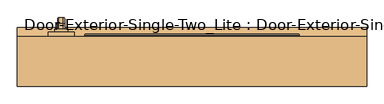
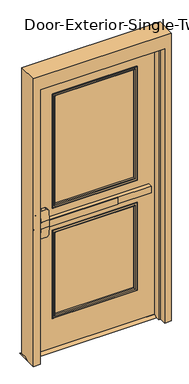
"""IFC4 building model written with IfcOpenShell, lengths in millimetres: door geometry, Door-Exterior-Single-Two_Lite : Door-Exterior-Single-Two_Lite."""

from ifc_helpers import new_model, si_unit, point, frame, frame_2d, origin, place, context, project, spatial, polyline, circle_curve, ellipse_curve, trimmed, segment, composite_curve, outline, extrude, faceted_brep, source, transform, mapped, element, save
from ifc_brep_helpers import plane_surface, cylinder_surface, revolved_surface, advanced_brep


def door_exterior_single_two_lite_door_exterior_single_two_lite_36a17ea7(model_context):
    return source(origin(), model_context, "Body", "SolidModel", [
        extrude(outline(polyline([(38.1, 12.7), (82.55, 12.7), (107.95, 0.0), (12.7, 0.0), (38.1, 12.7)])), frame((-508.0, 0.0, 0.0), z_axis=(1.0, 0.0, 0.0), x_axis=(0.0, 1.0, 0.0)), (0.0, 0.0, 1.0), 1016.0),
        extrude(outline(polyline([(150.2833333, 0.0), (-349.25, 0.0), (-349.25, 6.35), (150.2833333, 6.35), (150.2833333, 0.0)])), frame((0.0, 0.0, 990.6), z_axis=(0.0, 0.0, 1.0), x_axis=(1.0, 0.0, 0.0)), (0.0, 0.0, 1.0), 50.8),
        advanced_brep(
        [(-412.75, 6.35, 1041.4), (-412.75, 6.35, 990.6), (-349.25, 6.35, 990.6), (400.05, 6.35, 990.6), (400.05, 6.35, 1041.4), (-349.25, 6.35, 1041.4), (400.05, 38.1, 1041.4), (400.05, 38.1, 990.6), (-349.25, 38.1, 990.6), (-349.25, 38.1, 927.1), (-368.3, 38.1, 908.05), (-393.7, 38.1, 908.05), (-412.75, 38.1, 927.1), (-412.75, 38.1, 1104.9), (-393.7, 38.1, 1123.95), (-368.3, 38.1, 1123.95), (-349.25, 38.1, 1104.9), (-349.25, 38.1, 1041.4), (-349.25, 9.5252467, 1041.4), (-412.75, 9.5252467, 1041.4), (-412.75, 14.5354269, 1104.9), (-412.75, 14.5354269, 927.1), (-412.75, 9.5252467, 990.6), (-349.25, 9.5252467, 990.6), (-349.25, 14.5354269, 927.1), (-349.25, 14.5354269, 1104.9), (-393.7, 16.038481, 1123.95), (-368.3, 16.038481, 1123.95), (-368.3, 16.038481, 908.05), (-393.7, 16.038481, 908.05)],
        [
            (0, 1),
            (1, 2),
            (2, 3),
            (3, 4),
            (4, 5),
            (5, 0),
            (6, 7),
            (7, 8),
            (8, 9),
            (9, 10, circle_curve(frame((-368.3, 38.1, 927.1), z_axis=(0.0, 1.0, 0.0), x_axis=(1.0, 0.0, 0.0)), 19.05)),
            (10, 11),
            (11, 12, circle_curve(frame((-393.7, 38.1, 927.1), z_axis=(0.0, 1.0, 0.0), x_axis=(1.0, 0.0, 0.0)), 19.05)),
            (12, 13),
            (13, 14, circle_curve(frame((-393.7, 38.1, 1104.9), z_axis=(0.0, 1.0, 0.0), x_axis=(1.0, 0.0, 0.0)), 19.05)),
            (14, 15),
            (15, 16, circle_curve(frame((-368.3, 38.1, 1104.9), z_axis=(0.0, 1.0, 0.0), x_axis=(1.0, 0.0, 0.0)), 19.05)),
            (16, 17),
            (17, 6),
            (4, 6),
            (17, 18),
            (18, 19),
            (19, 0),
            (19, 20),
            (20, 13),
            (12, 21),
            (21, 22),
            (22, 1),
            (7, 3),
            (22, 23),
            (23, 8),
            (23, 24),
            (24, 9),
            (16, 25),
            (25, 18),
            (14, 26),
            (26, 27),
            (27, 15),
            (10, 28),
            (28, 29),
            (29, 11),
            (24, 28, ellipse_curve(frame((-368.3, 14.5354269, 927.1), z_axis=(0.0, 0.9969018152893365, 0.07865602756830282), x_axis=(0.0, -0.07865602756830208, 0.9969018152893365)), 19.1092038, 19.05)),
            (27, 25, ellipse_curve(frame((-368.3, 14.5354269, 1104.9), z_axis=(0.0, 0.9969018152893376, -0.07865602756828934), x_axis=(0.0, -0.078656027568288, -0.9969018152893377)), 19.1092038, 19.05)),
            (20, 26, ellipse_curve(frame((-393.7, 14.5354269, 1104.9), z_axis=(0.0, 0.9969018152893376, -0.07865602756828934), x_axis=(0.0, -0.078656027568288, -0.9969018152893377)), 19.1092038, 19.05)),
            (29, 21, ellipse_curve(frame((-393.7, 14.5354269, 927.1), z_axis=(0.0, 0.9969018152893365, 0.07865602756830282), x_axis=(0.0, -0.07865602756830208, 0.9969018152893365)), 19.1092038, 19.05)),
        ],
        [
            plane_surface(frame((-412.75, 6.35, 1041.4), z_axis=(0.0, -1.0, 0.0), x_axis=(-1.0, 0.0, 0.0))),
            plane_surface(frame((-412.75, 38.1, 1041.4), z_axis=(0.0, 1.0, 0.0), x_axis=(1.0, 0.0, 0.0))),
            plane_surface(frame((400.05, 6.35, 1041.4), z_axis=(0.0, 0.0, 1.0), x_axis=(0.0, 1.0, 0.0))),
            plane_surface(frame((-412.75, 6.35, 1041.4), z_axis=(-1.0, 0.0, 0.0), x_axis=(0.0, 1.0, 0.0))),
            plane_surface(frame((-412.75, 6.35, 990.6), z_axis=(0.0, 0.0, -1.0), x_axis=(0.0, 1.0, 0.0))),
            plane_surface(frame((400.05, 6.35, 990.6), z_axis=(1.0, 0.0, 0.0), x_axis=(0.0, 1.0, 0.0))),
            plane_surface(frame((-349.25, 9.5252467, 927.1), z_axis=(1.0, 0.0, 0.0), x_axis=(0.0, 1.0, 0.0))),
            plane_surface(frame((-368.3, 9.5252467, 1123.95), z_axis=(0.0, 0.0, 1.0), x_axis=(0.0, 1.0, 0.0))),
            plane_surface(frame((-393.7, 9.5252467, 908.05), z_axis=(0.0, 0.0, -1.0), x_axis=(0.0, 1.0, 0.0))),
            cylinder_surface(frame((-368.3, 38.1, 927.1), z_axis=(0.0, -1.0, 0.0), x_axis=(1.0, 0.0, 0.0)), 19.05),
            cylinder_surface(frame((-368.3, 38.1, 1104.9), z_axis=(0.0, -1.0, 0.0), x_axis=(1.0, 0.0, 0.0)), 19.05),
            cylinder_surface(frame((-393.7, 38.1, 1104.9), z_axis=(0.0, -1.0, 0.0), x_axis=(1.0, 0.0, 0.0)), 19.05),
            cylinder_surface(frame((-393.7, 38.1, 927.1), z_axis=(0.0, -1.0, 0.0), x_axis=(1.0, 0.0, 0.0)), 19.05),
            plane_surface(frame((-349.25, 9.5252467, 1041.4), z_axis=(0.0, -0.9969018152893376, 0.07865602756828934), x_axis=(-1.0, 0.0, 0.0))),
            plane_surface(frame((-349.25, 16.038481, 908.05), z_axis=(0.0, -0.9969018152893365, -0.07865602756830282), x_axis=(-1.0, 0.0, 0.0))),
        ],
        [
            (0, [[1, 2, 3, 4, 5, 6]]),
            (1, [[7, 8, 9, 10, 11, 12, 13, 14, 15, 16, 17, 18]]),
            (2, [[19, -18, 20, 21, 22, -6, -5]]),
            (3, [[-1, -22, 23, 24, -13, 25, 26, 27]]),
            (4, [[28, -3, -2, -27, 29, 30, -8]]),
            (5, [[-4, -28, -7, -19]]),
            (6, [[-9, -30, 31, 32]]),
            (6, [[-17, 33, 34, -20]]),
            (7, [[-15, 35, 36, 37]]),
            (8, [[-11, 38, 39, 40]]),
            (9, [[-10, -32, 41, -38]]),
            (10, [[-16, -37, 42, -33]]),
            (11, [[-14, -24, 43, -35]]),
            (12, [[-12, -40, 44, -25]]),
            (13, [[-21, -34, -42, -36, -43, -23]]),
            (14, [[-26, -44, -39, -41, -31, -29]]),
        ],
    ),
        advanced_brep(
        [(-391.0, 95.25, 1017.190625), (-391.0, 95.25, 1014.809375), (-387.428125, 95.25, 1011.2375), (-374.5715406, 95.25, 1011.2375), (-371.0, 95.25, 1014.8090406), (-371.0, 95.25, 1017.190625), (-374.571875, 95.25, 1020.7625), (-387.428125, 95.25, 1020.7625), (-391.0, 95.25, 887.809375), (-387.428125, 95.25, 884.2375), (-374.571875, 95.25, 884.2375), (-371.0, 95.25, 887.809375), (-371.0, 95.25, 890.1909594), (-374.5715406, 95.25, 893.7625), (-387.428125, 95.25, 893.7625), (-391.0, 95.25, 890.190625), (-391.0, 120.65, 1017.190625), (-391.0, 134.540625, 1003.3), (-391.0, 134.540625, 901.7), (-391.0, 120.65, 887.809375), (-391.0, 120.65, 890.190625), (-391.0, 132.159375, 901.7), (-391.0, 132.159375, 1003.3), (-391.0, 120.65, 1014.809375), (-387.428125, 120.65, 1011.2375), (-374.5715406, 120.65, 1011.2375), (-371.0, 120.65, 1014.8090406), (-371.0, 132.1590406, 1003.3), (-371.0, 132.1590406, 901.7), (-371.0, 120.65, 890.1909594), (-371.0, 120.65, 887.809375), (-371.0, 134.540625, 901.7), (-371.0, 134.540625, 1003.3), (-371.0, 120.65, 1017.190625), (-374.571875, 120.65, 1020.7625), (-387.428125, 120.65, 1020.7625), (-387.428125, 128.5875, 1003.3), (-374.5715406, 128.5875, 1003.3), (-374.571875, 138.1125, 1003.3), (-387.428125, 138.1125, 1003.3), (-387.428125, 128.5875, 901.7), (-374.5715406, 128.5875, 901.7), (-374.571875, 138.1125, 901.7), (-387.428125, 138.1125, 901.7), (-387.428125, 120.65, 893.7625), (-374.5715406, 120.65, 893.7625), (-374.571875, 120.65, 884.2375), (-387.428125, 120.65, 884.2375)],
        [
            (0, 1),
            (1, 2, circle_curve(frame((-387.428125, 95.25, 1014.809375), z_axis=(0.0, -1.0, 0.0), x_axis=(0.0, 0.0, 1.0)), 3.571875)),
            (2, 3),
            (3, 4, circle_curve(frame((-374.5715406, 95.25, 1014.8090406), z_axis=(0.0, -1.0, 0.0), x_axis=(0.0, 0.0, 1.0)), 3.5715406)),
            (4, 5),
            (5, 6, circle_curve(frame((-374.571875, 95.25, 1017.190625), z_axis=(0.0, -1.0, 0.0), x_axis=(0.0, 0.0, 1.0)), 3.571875)),
            (6, 7),
            (7, 0, circle_curve(frame((-387.428125, 95.25, 1017.190625), z_axis=(0.0, -1.0, 0.0), x_axis=(0.0, 0.0, 1.0)), 3.571875)),
            (8, 9, circle_curve(frame((-387.428125, 95.25, 887.809375), z_axis=(0.0, -1.0, 0.0), x_axis=(0.0, 0.0, -1.0)), 3.571875)),
            (9, 10),
            (10, 11, circle_curve(frame((-374.571875, 95.25, 887.809375), z_axis=(0.0, -1.0, 0.0), x_axis=(0.0, 0.0, -1.0)), 3.571875)),
            (11, 12),
            (12, 13, circle_curve(frame((-374.5715406, 95.25, 890.1909594), z_axis=(0.0, -1.0, 0.0), x_axis=(0.0, 0.0, -1.0)), 3.5715406)),
            (13, 14),
            (14, 15, circle_curve(frame((-387.428125, 95.25, 890.190625), z_axis=(0.0, -1.0, 0.0), x_axis=(0.0, 0.0, -1.0)), 3.571875)),
            (15, 8),
            (0, 16),
            (16, 17, circle_curve(frame((-391.0, 120.65, 1003.3), z_axis=(-1.0, 0.0, 0.0), x_axis=(0.0, 0.0, 1.0)), 13.890625)),
            (17, 18),
            (18, 19, circle_curve(frame((-391.0, 120.65, 901.7), z_axis=(-1.0, 0.0, 0.0), x_axis=(0.0, 1.0, 0.0)), 13.890625)),
            (19, 8),
            (15, 20),
            (20, 21, circle_curve(frame((-391.0, 120.65, 901.7), z_axis=(1.0, 0.0, 0.0), x_axis=(0.0, 1.0, 0.0)), 11.509375)),
            (21, 22),
            (22, 23, circle_curve(frame((-391.0, 120.65, 1003.3), z_axis=(1.0, 0.0, 0.0), x_axis=(0.0, 0.0, 1.0)), 11.509375)),
            (23, 1),
            (23, 24, circle_curve(frame((-387.428125, 120.65, 1014.809375), z_axis=(0.0, -1.0, 0.0), x_axis=(0.0, 0.0, 1.0)), 3.571875)),
            (24, 2),
            (24, 25),
            (25, 3),
            (25, 26, circle_curve(frame((-374.5715406, 120.65, 1014.8090406), z_axis=(0.0, -1.0, 0.0), x_axis=(0.0, 0.0, 1.0)), 3.5715406)),
            (26, 4),
            (26, 27, circle_curve(frame((-371.0, 120.65, 1003.3), z_axis=(-1.0, 0.0, 0.0), x_axis=(0.0, 0.0, 1.0)), 11.5090406)),
            (27, 28),
            (28, 29, circle_curve(frame((-371.0, 120.65, 901.7), z_axis=(-1.0, 0.0, 0.0), x_axis=(0.0, 1.0, 0.0)), 11.5090406)),
            (29, 12),
            (11, 30),
            (30, 31, circle_curve(frame((-371.0, 120.65, 901.7), z_axis=(1.0, 0.0, 0.0), x_axis=(0.0, 1.0, 0.0)), 13.890625)),
            (31, 32),
            (32, 33, circle_curve(frame((-371.0, 120.65, 1003.3), z_axis=(1.0, 0.0, 0.0), x_axis=(0.0, 0.0, 1.0)), 13.890625)),
            (33, 5),
            (33, 34, circle_curve(frame((-374.571875, 120.65, 1017.190625), z_axis=(0.0, -1.0, 0.0), x_axis=(0.0, 0.0, 1.0)), 3.571875)),
            (34, 6),
            (34, 35),
            (35, 7),
            (35, 16, circle_curve(frame((-387.428125, 120.65, 1017.190625), z_axis=(0.0, -1.0, 0.0), x_axis=(0.0, 0.0, 1.0)), 3.571875)),
            (36, 24, circle_curve(frame((-387.428125, 120.65, 1003.3), z_axis=(1.0, 0.0, 0.0), x_axis=(0.0, 0.0, 1.0)), 7.9375)),
            (22, 36, circle_curve(frame((-387.428125, 132.159375, 1003.3), z_axis=(0.0, 0.0, 1.0), x_axis=(0.0, 1.0, 0.0)), 3.571875)),
            (37, 25, circle_curve(frame((-374.5715406, 120.65, 1003.3), z_axis=(1.0, 0.0, 0.0), x_axis=(0.0, 0.0, 1.0)), 7.9375)),
            (36, 37),
            (37, 27, circle_curve(frame((-374.5715406, 132.1590406, 1003.3), z_axis=(0.0, 0.0, 1.0), x_axis=(0.0, 1.0, 0.0)), 3.5715406)),
            (38, 34, circle_curve(frame((-374.571875, 120.65, 1003.3), z_axis=(1.0, 0.0, 0.0), x_axis=(0.0, 0.0, 1.0)), 17.4625)),
            (32, 38, circle_curve(frame((-374.571875, 134.540625, 1003.3), z_axis=(0.0, 0.0, 1.0), x_axis=(0.0, 1.0, 0.0)), 3.571875)),
            (39, 35, circle_curve(frame((-387.428125, 120.65, 1003.3), z_axis=(1.0, 0.0, 0.0), x_axis=(0.0, 0.0, 1.0)), 17.4625)),
            (38, 39),
            (39, 17, circle_curve(frame((-387.428125, 134.540625, 1003.3), z_axis=(0.0, 0.0, 1.0), x_axis=(0.0, 1.0, 0.0)), 3.571875)),
            (21, 40, circle_curve(frame((-387.428125, 132.159375, 901.7), z_axis=(0.0, 0.0, 1.0), x_axis=(0.0, 1.0, 0.0)), 3.571875)),
            (40, 36),
            (40, 41),
            (41, 37),
            (41, 28, circle_curve(frame((-374.5715406, 132.1590406, 901.7), z_axis=(0.0, 0.0, 1.0), x_axis=(0.0, 1.0, 0.0)), 3.5715406)),
            (31, 42, circle_curve(frame((-374.571875, 134.540625, 901.7), z_axis=(0.0, 0.0, 1.0), x_axis=(0.0, 1.0, 0.0)), 3.571875)),
            (42, 38),
            (42, 43),
            (43, 39),
            (43, 18, circle_curve(frame((-387.428125, 134.540625, 901.7), z_axis=(0.0, 0.0, 1.0), x_axis=(0.0, 1.0, 0.0)), 3.571875)),
            (44, 40, circle_curve(frame((-387.428125, 120.65, 901.7), z_axis=(1.0, 0.0, 0.0), x_axis=(0.0, 1.0, 0.0)), 7.9375)),
            (20, 44, circle_curve(frame((-387.428125, 120.65, 890.190625), z_axis=(0.0, 1.0, 0.0), x_axis=(0.0, 0.0, -1.0)), 3.571875)),
            (45, 41, circle_curve(frame((-374.5715406, 120.65, 901.7), z_axis=(1.0, 0.0, 0.0), x_axis=(0.0, 1.0, 0.0)), 7.9375)),
            (44, 45),
            (45, 29, circle_curve(frame((-374.5715406, 120.65, 890.1909594), z_axis=(0.0, 1.0, 0.0), x_axis=(0.0, 0.0, -1.0)), 3.5715406)),
            (46, 42, circle_curve(frame((-374.571875, 120.65, 901.7), z_axis=(1.0, 0.0, 0.0), x_axis=(0.0, 1.0, 0.0)), 17.4625)),
            (30, 46, circle_curve(frame((-374.571875, 120.65, 887.809375), z_axis=(0.0, 1.0, 0.0), x_axis=(0.0, 0.0, -1.0)), 3.571875)),
            (47, 43, circle_curve(frame((-387.428125, 120.65, 901.7), z_axis=(1.0, 0.0, 0.0), x_axis=(0.0, 1.0, 0.0)), 17.4625)),
            (46, 47),
            (47, 19, circle_curve(frame((-387.428125, 120.65, 887.809375), z_axis=(0.0, 1.0, 0.0), x_axis=(0.0, 0.0, -1.0)), 3.571875)),
            (14, 44),
            (13, 45),
            (10, 46),
            (9, 47),
        ],
        [
            plane_surface(frame((-381.0, 95.25, 1016.0), z_axis=(0.0, -1.0, 0.0), x_axis=(1.0, 0.0, 0.0))),
            plane_surface(frame((-381.0, 95.25, 889.0), z_axis=(0.0, -1.0, 0.0), x_axis=(1.0, 0.0, 0.0))),
            plane_surface(frame((-391.0, 95.25, 1017.190625), z_axis=(-1.0, 0.0, 0.0), x_axis=(0.0, 1.0, 0.0))),
            cylinder_surface(frame((-387.428125, 95.25, 1014.809375), z_axis=(0.0, -1.0, 0.0), x_axis=(0.0, 0.0, 1.0)), 3.571875),
            plane_surface(frame((-387.428125, 95.25, 1011.2375), z_axis=(0.0, 0.0, -1.0), x_axis=(0.0, 1.0, 0.0))),
            cylinder_surface(frame((-374.5715406, 95.25, 1014.8090406), z_axis=(0.0, -1.0, 0.0), x_axis=(0.0, 0.0, 1.0)), 3.5715406),
            plane_surface(frame((-371.0, 95.25, 1014.8090406), z_axis=(1.0, 0.0, 0.0), x_axis=(0.0, 1.0, 0.0))),
            cylinder_surface(frame((-374.571875, 95.25, 1017.190625), z_axis=(0.0, -1.0, 0.0), x_axis=(0.0, 0.0, 1.0)), 3.571875),
            plane_surface(frame((-374.571875, 95.25, 1020.7625), z_axis=(0.0, 0.0, 1.0), x_axis=(0.0, 1.0, 0.0))),
            cylinder_surface(frame((-387.428125, 95.25, 1017.190625), z_axis=(0.0, -1.0, 0.0), x_axis=(0.0, 0.0, 1.0)), 3.571875),
            revolved_surface(trimmed(ellipse_curve(frame((-387.428125, 120.65, 1014.809375), z_axis=(0.0, -1.0, 0.0), x_axis=(0.0, 0.0, 1.0)), 3.571875, 3.571875), [point((-391.0, 120.65, 1014.809375))], [point((-387.428125, 120.65, 1011.2375))], True, "CARTESIAN"), (-381.0, 120.65, 1003.3), (-1.0, 0.0, 0.0)),
            revolved_surface(polyline([(-387.428125, 120.65, 1011.2375), (-374.5715406, 120.65, 1011.2375)]), (-381.0, 120.65, 1003.3), (-1.0, 0.0, 0.0)),
            revolved_surface(trimmed(ellipse_curve(frame((-374.5715406, 120.65, 1014.8090406), z_axis=(0.0, -1.0, 0.0), x_axis=(0.0, 0.0, 1.0)), 3.5715406, 3.5715406), [point((-374.5715406, 120.65, 1011.2375))], [point((-371.0, 120.65, 1014.8090406))], True, "CARTESIAN"), (-381.0, 120.65, 1003.3), (-1.0, 0.0, 0.0)),
            revolved_surface(trimmed(ellipse_curve(frame((-374.571875, 120.65, 1017.190625), z_axis=(0.0, -1.0, 0.0), x_axis=(0.0, 0.0, 1.0)), 3.571875, 3.571875), [point((-371.0, 120.65, 1017.190625))], [point((-374.571875, 120.65, 1020.7625))], True, "CARTESIAN"), (-381.0, 120.65, 1003.3), (-1.0, 0.0, 0.0)),
            cylinder_surface(frame((-381.0, 120.65, 1003.3), z_axis=(-1.0, 0.0, 0.0), x_axis=(0.0, 0.0, 1.0)), 17.4625),
            revolved_surface(trimmed(ellipse_curve(frame((-387.428125, 120.65, 1017.190625), z_axis=(0.0, -1.0, 0.0), x_axis=(0.0, 0.0, 1.0)), 3.571875, 3.571875), [point((-387.428125, 120.65, 1020.7625))], [point((-391.0, 120.65, 1017.190625))], True, "CARTESIAN"), (-381.0, 120.65, 1003.3), (-1.0, 0.0, 0.0)),
            cylinder_surface(frame((-387.428125, 132.159375, 1003.3), z_axis=(0.0, 0.0, 1.0), x_axis=(0.0, 1.0, 0.0)), 3.571875),
            plane_surface(frame((-387.428125, 128.5875, 1003.3), z_axis=(0.0, -1.0, 0.0), x_axis=(0.0, 0.0, -1.0))),
            cylinder_surface(frame((-374.5715406, 132.1590406, 1003.3), z_axis=(0.0, 0.0, 1.0), x_axis=(0.0, 1.0, 0.0)), 3.5715406),
            cylinder_surface(frame((-374.571875, 134.540625, 1003.3), z_axis=(0.0, 0.0, 1.0), x_axis=(0.0, 1.0, 0.0)), 3.571875),
            plane_surface(frame((-374.571875, 138.1125, 1003.3), z_axis=(0.0, 1.0, 0.0), x_axis=(0.0, 0.0, -1.0))),
            cylinder_surface(frame((-387.428125, 134.540625, 1003.3), z_axis=(0.0, 0.0, 1.0), x_axis=(0.0, 1.0, 0.0)), 3.571875),
            revolved_surface(trimmed(ellipse_curve(frame((-387.428125, 132.159375, 901.7), z_axis=(0.0, 0.0, 1.0), x_axis=(0.0, 1.0, 0.0)), 3.571875, 3.571875), [point((-391.0, 132.159375, 901.7))], [point((-387.428125, 128.5875, 901.7))], True, "CARTESIAN"), (-381.0, 120.65, 901.7), (-1.0, 0.0, 0.0)),
            revolved_surface(polyline([(-387.428125, 128.5875, 901.7), (-374.5715406, 128.5875, 901.7)]), (-381.0, 120.65, 901.7), (-1.0, 0.0, 0.0)),
            revolved_surface(trimmed(ellipse_curve(frame((-374.5715406, 132.1590406, 901.7), z_axis=(0.0, 0.0, 1.0), x_axis=(0.0, 1.0, 0.0)), 3.5715406, 3.5715406), [point((-374.5715406, 128.5875, 901.7))], [point((-371.0, 132.1590406, 901.7))], True, "CARTESIAN"), (-381.0, 120.65, 901.7), (-1.0, 0.0, 0.0)),
            revolved_surface(trimmed(ellipse_curve(frame((-374.571875, 134.540625, 901.7), z_axis=(0.0, 0.0, 1.0), x_axis=(0.0, 1.0, 0.0)), 3.571875, 3.571875), [point((-371.0, 134.540625, 901.7))], [point((-374.571875, 138.1125, 901.7))], True, "CARTESIAN"), (-381.0, 120.65, 901.7), (-1.0, 0.0, 0.0)),
            cylinder_surface(frame((-381.0, 120.65, 901.7), z_axis=(-1.0, 0.0, 0.0), x_axis=(0.0, 1.0, 0.0)), 17.4625),
            revolved_surface(trimmed(ellipse_curve(frame((-387.428125, 134.540625, 901.7), z_axis=(0.0, 0.0, 1.0), x_axis=(0.0, 1.0, 0.0)), 3.571875, 3.571875), [point((-387.428125, 138.1125, 901.7))], [point((-391.0, 134.540625, 901.7))], True, "CARTESIAN"), (-381.0, 120.65, 901.7), (-1.0, 0.0, 0.0)),
            cylinder_surface(frame((-387.428125, 120.65, 890.190625), z_axis=(0.0, 1.0, 0.0), x_axis=(0.0, 0.0, -1.0)), 3.571875),
            plane_surface(frame((-387.428125, 120.65, 893.7625), z_axis=(0.0, 0.0, 1.0), x_axis=(0.0, -1.0, 0.0))),
            cylinder_surface(frame((-374.5715406, 120.65, 890.1909594), z_axis=(0.0, 1.0, 0.0), x_axis=(0.0, 0.0, -1.0)), 3.5715406),
            cylinder_surface(frame((-374.571875, 120.65, 887.809375), z_axis=(0.0, 1.0, 0.0), x_axis=(0.0, 0.0, -1.0)), 3.571875),
            plane_surface(frame((-374.571875, 120.65, 884.2375), z_axis=(0.0, 0.0, -1.0), x_axis=(0.0, -1.0, 0.0))),
            cylinder_surface(frame((-387.428125, 120.65, 887.809375), z_axis=(0.0, 1.0, 0.0), x_axis=(0.0, 0.0, -1.0)), 3.571875),
        ],
        [
            (0, [[1, 2, 3, 4, 5, 6, 7, 8]]),
            (1, [[9, 10, 11, 12, 13, 14, 15, 16]]),
            (2, [[-1, 17, 18, 19, 20, 21, -16, 22, 23, 24, 25, 26]]),
            (3, [[-2, -26, 27, 28]]),
            (4, [[-3, -28, 29, 30]]),
            (5, [[-4, -30, 31, 32]]),
            (6, [[-5, -32, 33, 34, 35, 36, -12, 37, 38, 39, 40, 41]]),
            (7, [[-6, -41, 42, 43]]),
            (8, [[-7, -43, 44, 45]]),
            (9, [[-8, -45, 46, -17]]),
            (10, [[47, -27, -25, 48]]),
            (11, [[49, -29, -47, 50]]),
            (12, [[-33, -31, -49, 51]]),
            (13, [[52, -42, -40, 53]]),
            (14, [[54, -44, -52, 55]]),
            (15, [[-18, -46, -54, 56]]),
            (16, [[-48, -24, 57, 58]]),
            (17, [[-50, -58, 59, 60]]),
            (18, [[-51, -60, 61, -34]]),
            (19, [[-53, -39, 62, 63]]),
            (20, [[-55, -63, 64, 65]]),
            (21, [[-56, -65, 66, -19]]),
            (22, [[67, -57, -23, 68]]),
            (23, [[69, -59, -67, 70]]),
            (24, [[-35, -61, -69, 71]]),
            (25, [[72, -62, -38, 73]]),
            (26, [[74, -64, -72, 75]]),
            (27, [[-20, -66, -74, 76]]),
            (28, [[-68, -22, -15, 77]]),
            (29, [[-70, -77, -14, 78]]),
            (30, [[-71, -78, -13, -36]]),
            (31, [[-73, -37, -11, 79]]),
            (32, [[-75, -79, -10, 80]]),
            (33, [[-76, -80, -9, -21]]),
        ],
    ),
        extrude(outline(composite_curve([segment(trimmed(circle_curve(frame_2d((1117.6, -381.0)), 19.0), [point((1117.6, -400.0))], [point((1117.6, -362.0))], False, "CARTESIAN"), True, "CONTINUOUS"), segment(trimmed(circle_curve(frame_2d((1117.6, -381.0)), 19.0), [point((1117.6, -362.0))], [point((1117.6, -400.0))], False, "CARTESIAN"), True, "CONTINUOUS")], self_intersect=False)), frame((0.0, 95.25, 0.0), z_axis=(0.0, 1.0, 0.0), x_axis=(0.0, 0.0, 1.0)), (0.0, 0.0, 1.0), 8.73125),
        extrude(outline(composite_curve([segment(trimmed(circle_curve(frame_2d((1113.0338574, -381.0)), 89.3016225), [point((1193.8, -342.9))], [point((1193.8, -419.1))], False, "CARTESIAN"), True, "CONTINUOUS"), segment(polyline([(1193.8, -419.1), (838.2, -419.1)]), True, "CONTINUOUS"), segment(trimmed(circle_curve(frame_2d((918.9661426, -381.0)), 89.3016225), [point((838.2, -419.1))], [point((838.2, -342.9))], False, "CARTESIAN"), True, "CONTINUOUS"), segment(polyline([(838.2, -342.9), (1193.8, -342.9)]), True, "CONTINUOUS")], self_intersect=False)), frame((0.0, 82.55, 0.0), z_axis=(0.0, 1.0, 0.0), x_axis=(0.0, 0.0, 1.0)), (0.0, 0.0, 1.0), 12.7),
        faceted_brep([(457.2, 33.3375, 0.0), (457.2, 82.55, 0.0), (508.0, 82.55, 0.0), (508.0, -63.5, 0.0), (457.2, -63.5, 0.0), (457.2, -14.2875, 0.0), (441.325, -14.2875, 0.0), (441.325, 33.3375, 0.0), (457.2, 33.3375, 2133.6), (457.2, 82.55, 2133.6), (-457.2, 82.55, 2133.6), (-457.2, 82.55, 0.0), (-508.0, 82.55, 0.0), (-508.0, 82.55, 2235.2), (508.0, 82.55, 2235.2), (508.0, -63.5, 2235.2), (-508.0, -63.5, 2235.2), (-508.0, -63.5, 0.0), (-457.2, -63.5, 0.0), (-457.2, -63.5, 2133.6), (457.2, -63.5, 2133.6), (457.2, -14.2875, 2133.6), (-457.2, -14.2875, 2133.6), (-457.2, -14.2875, 0.0), (-441.325, -14.2875, 0.0), (-441.325, -14.2875, 2117.725), (441.325, -14.2875, 2117.725), (441.325, 33.3375, 2117.725), (-441.325, 33.3375, 2117.725), (-441.325, 33.3375, 0.0), (-457.2, 33.3375, 0.0), (-457.2, 33.3375, 2133.6)], [[[0, 1, 2, 3, 4, 5, 6, 7]], [[1, 0, 8, 9]], [[2, 1, 9, 10, 11, 12, 13, 14]], [[3, 2, 14, 15]], [[4, 3, 15, 16, 17, 18, 19, 20]], [[5, 4, 20, 21]], [[6, 5, 21, 22, 23, 24, 25, 26]], [[7, 6, 26, 27]], [[0, 7, 27, 28, 29, 30, 31, 8]], [[9, 8, 31, 10]], [[20, 19, 22, 21]], [[26, 25, 28, 27]], [[12, 11, 30, 29, 24, 23, 18, 17]], [[11, 10, 31, 30]], [[13, 12, 17, 16]], [[19, 18, 23, 22]], [[25, 24, 29, 28]], [[15, 14, 13, 16]]]),
        extrude(outline(polyline([(2133.6, -457.2), (12.7, -457.2), (12.7, 457.2), (2133.6, 457.2), (2133.6, -457.2)]), holes=[polyline([(1981.2, -304.8), (1981.2, 304.8), (1111.25, 304.8), (1111.25, -304.8), (1981.2, -304.8)]), polyline([(920.75, -304.8), (920.75, 304.8), (254.0, 304.8), (254.0, -304.8), (920.75, -304.8)])]), frame((0.0, 38.1, 0.0), z_axis=(0.0, 1.0, 0.0), x_axis=(0.0, 0.0, 1.0)), (0.0, 0.0, 1.0), 44.45),
        extrude(outline(polyline([(304.8, 50.8), (-304.8, 50.8), (-304.8, 69.85), (304.8, 69.85), (304.8, 50.8)])), frame((0.0, 0.0, 1111.25), z_axis=(0.0, 0.0, 1.0), x_axis=(1.0, 0.0, 0.0)), (0.0, 0.0, 1.0), 869.95),
        extrude(outline(polyline([(304.8, 50.8), (-304.8, 50.8), (-304.8, 69.85), (304.8, 69.85), (304.8, 50.8)])), frame((0.0, 0.0, 254.0), z_axis=(0.0, 0.0, 1.0), x_axis=(1.0, 0.0, 0.0)), (0.0, 0.0, 1.0), 666.75),
        advanced_brep(
        [(304.8, 50.8, 920.75), (304.8, 38.1, 920.75), (304.8, 38.1, 254.0), (304.8, 50.8, 254.0), (292.8, 37.1, 908.75), (292.8, 50.8, 908.75), (292.8, 50.8, 266.0), (292.8, 37.1, 266.0), (297.8, 32.1, 913.75), (297.8, 32.1, 261.0), (312.8, 34.1, 928.75), (310.8, 32.1, 926.75), (310.8, 32.1, 248.0), (312.8, 34.1, 246.0), (312.8, 38.1, 928.75), (312.8, 38.1, 246.0), (-304.8, 38.1, 254.0), (-304.8, 50.8, 254.0), (-292.8, 50.8, 266.0), (-292.8, 37.1, 266.0), (-297.8, 32.1, 261.0), (-310.8, 32.1, 248.0), (-312.8, 34.1, 246.0), (-312.8, 38.1, 246.0), (-304.8, 38.1, 920.75), (-304.8, 50.8, 920.75), (-292.8, 50.8, 908.75), (-292.8, 37.1, 908.75), (-297.8, 32.1, 913.75), (-310.8, 32.1, 926.75), (-312.8, 34.1, 928.75), (-312.8, 38.1, 928.75)],
        [
            (0, 1),
            (1, 2),
            (2, 3),
            (3, 0),
            (4, 5),
            (5, 6),
            (6, 7),
            (7, 4),
            (8, 4, ellipse_curve(frame((297.8, 37.1, 913.75), z_axis=(0.7071067811865475, 0.0, -0.7071067811865475), x_axis=(0.7071067811865474, 0.0, 0.7071067811865476)), 7.0710678, 5.0)),
            (7, 9, ellipse_curve(frame((297.8, 37.1, 261.0), z_axis=(0.7071067811865475, 0.0, 0.7071067811865475), x_axis=(-0.7071067811865474, 0.0, 0.7071067811865476)), 7.0710678, 5.0)),
            (9, 8),
            (10, 11, ellipse_curve(frame((310.8, 34.1, 926.75), z_axis=(0.7071067811865475, 0.0, -0.7071067811865475), x_axis=(0.7071067811865474, 0.0, 0.7071067811865476)), 2.8284271, 2.0)),
            (11, 12),
            (12, 13, ellipse_curve(frame((310.8, 34.1, 248.0), z_axis=(0.7071067811865475, 0.0, 0.7071067811865475), x_axis=(-0.7071067811865474, 0.0, 0.7071067811865476)), 2.8284271, 2.0)),
            (13, 10),
            (14, 10),
            (13, 15),
            (15, 14),
            (2, 16),
            (16, 17),
            (17, 3),
            (6, 18),
            (18, 19),
            (19, 7),
            (19, 20, ellipse_curve(frame((-297.8, 37.1, 261.0), z_axis=(0.7071067811865475, 0.0, -0.7071067811865475), x_axis=(0.7071067811865476, 0.0, 0.7071067811865474)), 7.0710678, 5.0)),
            (20, 9),
            (12, 21),
            (21, 22, ellipse_curve(frame((-310.8, 34.1, 248.0), z_axis=(0.7071067811865475, 0.0, -0.7071067811865475), x_axis=(0.7071067811865476, 0.0, 0.7071067811865474)), 2.8284271, 2.0)),
            (22, 13),
            (22, 23),
            (23, 15),
            (16, 24),
            (24, 25),
            (25, 17),
            (18, 26),
            (26, 27),
            (27, 19),
            (27, 28, ellipse_curve(frame((-297.8, 37.1, 913.75), z_axis=(-0.7071067811865475, 0.0, -0.7071067811865475), x_axis=(0.7071067811865474, 0.0, -0.7071067811865476)), 7.0710678, 5.0)),
            (28, 20),
            (21, 29),
            (29, 30, ellipse_curve(frame((-310.8, 34.1, 926.75), z_axis=(-0.7071067811865475, 0.0, -0.7071067811865475), x_axis=(0.7071067811865474, 0.0, -0.7071067811865476)), 2.8284271, 2.0)),
            (30, 22),
            (30, 31),
            (31, 23),
            (31, 14),
            (1, 24),
            (0, 25),
            (5, 26),
            (4, 27),
            (8, 28),
            (11, 29),
            (10, 30),
        ],
        [
            plane_surface(frame((304.8, 38.1, 920.75), z_axis=(1.0, 0.0, 0.0), x_axis=(0.0, 0.0, -1.0))),
            plane_surface(frame((292.8, 50.8, 908.75), z_axis=(-1.0, 0.0, 0.0), x_axis=(0.0, 0.0, -1.0))),
            cylinder_surface(frame((297.8, 37.1, 920.75), z_axis=(0.0, 0.0, 1.0), x_axis=(1.0, 0.0, 0.0)), 5.0),
            cylinder_surface(frame((310.8, 34.1, 920.75), z_axis=(0.0, 0.0, 1.0), x_axis=(1.0, 0.0, 0.0)), 2.0),
            plane_surface(frame((312.8, 34.1, 928.75), z_axis=(1.0, 0.0, 0.0), x_axis=(0.0, 0.0, -1.0))),
            plane_surface(frame((304.8, 38.1, 254.0), z_axis=(0.0, 0.0, -1.0), x_axis=(-1.0, 0.0, 0.0))),
            plane_surface(frame((292.8, 50.8, 266.0), z_axis=(0.0, 0.0, 1.0), x_axis=(-1.0, 0.0, 0.0))),
            cylinder_surface(frame((304.8, 37.1, 261.0), z_axis=(1.0, 0.0, 0.0), x_axis=(0.0, 0.0, -1.0)), 5.0),
            cylinder_surface(frame((304.8, 34.1, 248.0), z_axis=(1.0, 0.0, 0.0), x_axis=(0.0, 0.0, -1.0)), 2.0),
            plane_surface(frame((312.8, 34.1, 246.0), z_axis=(0.0, 0.0, -1.0), x_axis=(-1.0, 0.0, 0.0))),
            plane_surface(frame((-304.8, 38.1, 254.0), z_axis=(-1.0, 0.0, 0.0), x_axis=(0.0, 0.0, 1.0))),
            plane_surface(frame((-292.8, 50.8, 266.0), z_axis=(1.0, 0.0, 0.0), x_axis=(0.0, 0.0, 1.0))),
            cylinder_surface(frame((-297.8, 37.1, 254.0), z_axis=(0.0, 0.0, -1.0), x_axis=(-1.0, 0.0, 0.0)), 5.0),
            cylinder_surface(frame((-310.8, 34.1, 254.0), z_axis=(0.0, 0.0, -1.0), x_axis=(-1.0, 0.0, 0.0)), 2.0),
            plane_surface(frame((-312.8, 34.1, 246.0), z_axis=(-1.0, 0.0, 0.0), x_axis=(0.0, 0.0, 1.0))),
            plane_surface(frame((-312.8, 38.1, 928.75), z_axis=(0.0, 1.0, 0.0), x_axis=(1.0, 0.0, 0.0))),
            plane_surface(frame((-304.8, 38.1, 920.75), z_axis=(0.0, 0.0, 1.0), x_axis=(1.0, 0.0, 0.0))),
            plane_surface(frame((-304.8, 50.8, 920.75), z_axis=(0.0, 1.0, 0.0), x_axis=(1.0, 0.0, 0.0))),
            plane_surface(frame((-292.8, 50.8, 908.75), z_axis=(0.0, 0.0, -1.0), x_axis=(1.0, 0.0, 0.0))),
            cylinder_surface(frame((-304.8, 37.1, 913.75), z_axis=(-1.0, 0.0, 0.0), x_axis=(0.0, 0.0, 1.0)), 5.0),
            plane_surface(frame((-297.8, 32.1, 913.75), z_axis=(0.0, -1.0, 0.0), x_axis=(1.0, 0.0, 0.0))),
            cylinder_surface(frame((-304.8, 34.1, 926.75), z_axis=(-1.0, 0.0, 0.0), x_axis=(0.0, 0.0, 1.0)), 2.0),
            plane_surface(frame((-312.8, 34.1, 928.75), z_axis=(0.0, 0.0, 1.0), x_axis=(1.0, 0.0, 0.0))),
        ],
        [
            (0, [[1, 2, 3, 4]]),
            (1, [[5, 6, 7, 8]]),
            (2, [[9, -8, 10, 11]]),
            (3, [[12, 13, 14, 15]]),
            (4, [[16, -15, 17, 18]]),
            (5, [[-3, 19, 20, 21]]),
            (6, [[-7, 22, 23, 24]]),
            (7, [[-10, -24, 25, 26]]),
            (8, [[-14, 27, 28, 29]]),
            (9, [[-17, -29, 30, 31]]),
            (10, [[-20, 32, 33, 34]]),
            (11, [[-23, 35, 36, 37]]),
            (12, [[-25, -37, 38, 39]]),
            (13, [[-28, 40, 41, 42]]),
            (14, [[-30, -42, 43, 44]]),
            (15, [[-31, -44, 45, -18], [46, -32, -19, -2]]),
            (16, [[-33, -46, -1, 47]]),
            (17, [[-21, -34, -47, -4], [48, -35, -22, -6]]),
            (18, [[-36, -48, -5, 49]]),
            (19, [[-38, -49, -9, 50]]),
            (20, [[51, -40, -27, -13], [-26, -39, -50, -11]]),
            (21, [[-41, -51, -12, 52]]),
            (22, [[-43, -52, -16, -45]]),
        ],
    ),
        advanced_brep(
        [(-304.8, 69.85, 920.75), (-304.8, 82.55, 920.75), (-304.8, 82.55, 254.0), (-304.8, 69.85, 254.0), (-292.8, 83.55, 908.75), (-292.8, 69.85, 908.75), (-292.8, 69.85, 266.0), (-292.8, 83.55, 266.0), (-297.8, 88.55, 913.75), (-297.8, 88.55, 261.0), (-312.8, 86.55, 928.75), (-310.8, 88.55, 926.75), (-310.8, 88.55, 248.0), (-312.8, 86.55, 246.0), (-312.8, 82.55, 928.75), (-312.8, 82.55, 246.0), (304.8, 82.55, 254.0), (304.8, 69.85, 254.0), (292.8, 69.85, 266.0), (292.8, 83.55, 266.0), (297.8, 88.55, 261.0), (310.8, 88.55, 248.0), (312.8, 86.55, 246.0), (312.8, 82.55, 246.0), (304.8, 82.55, 920.75), (304.8, 69.85, 920.75), (292.8, 69.85, 908.75), (292.8, 83.55, 908.75), (297.8, 88.55, 913.75), (310.8, 88.55, 926.75), (312.8, 86.55, 928.75), (312.8, 82.55, 928.75)],
        [
            (0, 1),
            (1, 2),
            (2, 3),
            (3, 0),
            (4, 5),
            (5, 6),
            (6, 7),
            (7, 4),
            (8, 4, ellipse_curve(frame((-297.8, 83.55, 913.75), z_axis=(-0.7071067811865475, 0.0, -0.7071067811865475), x_axis=(-0.7071067811865474, 0.0, 0.7071067811865476)), 7.0710678, 5.0)),
            (7, 9, ellipse_curve(frame((-297.8, 83.55, 261.0), z_axis=(-0.7071067811865475, 0.0, 0.7071067811865475), x_axis=(0.7071067811865474, 0.0, 0.7071067811865476)), 7.0710678, 5.0)),
            (9, 8),
            (10, 11, ellipse_curve(frame((-310.8, 86.55, 926.75), z_axis=(-0.7071067811865475, 0.0, -0.7071067811865475), x_axis=(-0.7071067811865474, 0.0, 0.7071067811865476)), 2.8284271, 2.0)),
            (11, 12),
            (12, 13, ellipse_curve(frame((-310.8, 86.55, 248.0), z_axis=(-0.7071067811865475, 0.0, 0.7071067811865475), x_axis=(0.7071067811865474, 0.0, 0.7071067811865476)), 2.8284271, 2.0)),
            (13, 10),
            (14, 10),
            (13, 15),
            (15, 14),
            (2, 16),
            (16, 17),
            (17, 3),
            (6, 18),
            (18, 19),
            (19, 7),
            (19, 20, ellipse_curve(frame((297.8, 83.55, 261.0), z_axis=(-0.7071067811865475, 0.0, -0.7071067811865475), x_axis=(-0.7071067811865476, 0.0, 0.7071067811865474)), 7.0710678, 5.0)),
            (20, 9),
            (12, 21),
            (21, 22, ellipse_curve(frame((310.8, 86.55, 248.0), z_axis=(-0.7071067811865475, 0.0, -0.7071067811865475), x_axis=(-0.7071067811865476, 0.0, 0.7071067811865474)), 2.8284271, 2.0)),
            (22, 13),
            (22, 23),
            (23, 15),
            (16, 24),
            (24, 25),
            (25, 17),
            (18, 26),
            (26, 27),
            (27, 19),
            (27, 28, ellipse_curve(frame((297.8, 83.55, 913.75), z_axis=(0.7071067811865475, 0.0, -0.7071067811865475), x_axis=(-0.7071067811865474, 0.0, -0.7071067811865476)), 7.0710678, 5.0)),
            (28, 20),
            (21, 29),
            (29, 30, ellipse_curve(frame((310.8, 86.55, 926.75), z_axis=(0.7071067811865475, 0.0, -0.7071067811865475), x_axis=(-0.7071067811865474, 0.0, -0.7071067811865476)), 2.8284271, 2.0)),
            (30, 22),
            (30, 31),
            (31, 23),
            (31, 14),
            (1, 24),
            (0, 25),
            (5, 26),
            (4, 27),
            (8, 28),
            (11, 29),
            (10, 30),
        ],
        [
            plane_surface(frame((-304.8, 82.55, 920.75), z_axis=(-1.0, 0.0, 0.0), x_axis=(0.0, 0.0, -1.0))),
            plane_surface(frame((-292.8, 69.85, 908.75), z_axis=(1.0, 0.0, 0.0), x_axis=(0.0, 0.0, -1.0))),
            cylinder_surface(frame((-297.8, 83.55, 920.75), z_axis=(0.0, 0.0, 1.0), x_axis=(-1.0, 0.0, 0.0)), 5.0),
            cylinder_surface(frame((-310.8, 86.55, 920.75), z_axis=(0.0, 0.0, 1.0), x_axis=(-1.0, 0.0, 0.0)), 2.0),
            plane_surface(frame((-312.8, 86.55, 928.75), z_axis=(-1.0, 0.0, 0.0), x_axis=(0.0, 0.0, -1.0))),
            plane_surface(frame((-304.8, 82.55, 254.0), z_axis=(0.0, 0.0, -1.0), x_axis=(1.0, 0.0, 0.0))),
            plane_surface(frame((-292.8, 69.85, 266.0), z_axis=(0.0, 0.0, 1.0), x_axis=(1.0, 0.0, 0.0))),
            cylinder_surface(frame((-304.8, 83.55, 261.0), z_axis=(-1.0, 0.0, 0.0), x_axis=(0.0, 0.0, -1.0)), 5.0),
            cylinder_surface(frame((-304.8, 86.55, 248.0), z_axis=(-1.0, 0.0, 0.0), x_axis=(0.0, 0.0, -1.0)), 2.0),
            plane_surface(frame((-312.8, 86.55, 246.0), z_axis=(0.0, 0.0, -1.0), x_axis=(1.0, 0.0, 0.0))),
            plane_surface(frame((304.8, 82.55, 254.0), z_axis=(1.0, 0.0, 0.0), x_axis=(0.0, 0.0, 1.0))),
            plane_surface(frame((292.8, 69.85, 266.0), z_axis=(-1.0, 0.0, 0.0), x_axis=(0.0, 0.0, 1.0))),
            cylinder_surface(frame((297.8, 83.55, 254.0), z_axis=(0.0, 0.0, -1.0), x_axis=(1.0, 0.0, 0.0)), 5.0),
            cylinder_surface(frame((310.8, 86.55, 254.0), z_axis=(0.0, 0.0, -1.0), x_axis=(1.0, 0.0, 0.0)), 2.0),
            plane_surface(frame((312.8, 86.55, 246.0), z_axis=(1.0, 0.0, 0.0), x_axis=(0.0, 0.0, 1.0))),
            plane_surface(frame((312.8, 82.55, 928.75), z_axis=(0.0, -1.0, 0.0), x_axis=(-1.0, 0.0, 0.0))),
            plane_surface(frame((304.8, 82.55, 920.75), z_axis=(0.0, 0.0, 1.0), x_axis=(-1.0, 0.0, 0.0))),
            plane_surface(frame((304.8, 69.85, 920.75), z_axis=(0.0, -1.0, 0.0), x_axis=(-1.0, 0.0, 0.0))),
            plane_surface(frame((292.8, 69.85, 908.75), z_axis=(0.0, 0.0, -1.0), x_axis=(-1.0, 0.0, 0.0))),
            cylinder_surface(frame((304.8, 83.55, 913.75), z_axis=(1.0, 0.0, 0.0), x_axis=(0.0, 0.0, 1.0)), 5.0),
            plane_surface(frame((297.8, 88.55, 913.75), z_axis=(0.0, 1.0, 0.0), x_axis=(-1.0, 0.0, 0.0))),
            cylinder_surface(frame((304.8, 86.55, 926.75), z_axis=(1.0, 0.0, 0.0), x_axis=(0.0, 0.0, 1.0)), 2.0),
            plane_surface(frame((312.8, 86.55, 928.75), z_axis=(0.0, 0.0, 1.0), x_axis=(-1.0, 0.0, 0.0))),
        ],
        [
            (0, [[1, 2, 3, 4]]),
            (1, [[5, 6, 7, 8]]),
            (2, [[9, -8, 10, 11]]),
            (3, [[12, 13, 14, 15]]),
            (4, [[16, -15, 17, 18]]),
            (5, [[-3, 19, 20, 21]]),
            (6, [[-7, 22, 23, 24]]),
            (7, [[-10, -24, 25, 26]]),
            (8, [[-14, 27, 28, 29]]),
            (9, [[-17, -29, 30, 31]]),
            (10, [[-20, 32, 33, 34]]),
            (11, [[-23, 35, 36, 37]]),
            (12, [[-25, -37, 38, 39]]),
            (13, [[-28, 40, 41, 42]]),
            (14, [[-30, -42, 43, 44]]),
            (15, [[-31, -44, 45, -18], [46, -32, -19, -2]]),
            (16, [[-33, -46, -1, 47]]),
            (17, [[-21, -34, -47, -4], [48, -35, -22, -6]]),
            (18, [[-36, -48, -5, 49]]),
            (19, [[-38, -49, -9, 50]]),
            (20, [[51, -40, -27, -13], [-26, -39, -50, -11]]),
            (21, [[-41, -51, -12, 52]]),
            (22, [[-43, -52, -16, -45]]),
        ],
    ),
        advanced_brep(
        [(-304.8, 50.8, 1111.25), (-304.8, 38.1, 1111.25), (-304.8, 38.1, 1981.2), (-304.8, 50.8, 1981.2), (-292.8, 37.1, 1123.25), (-292.8, 50.8, 1123.25), (-292.8, 50.8, 1969.2), (-292.8, 37.1, 1969.2), (-297.8, 32.1, 1118.25), (-297.8, 32.1, 1974.2), (-312.8, 34.1, 1103.25), (-310.8, 32.1, 1105.25), (-310.8, 32.1, 1987.2), (-312.8, 34.1, 1989.2), (-312.8, 38.1, 1103.25), (-312.8, 38.1, 1989.2), (304.8, 38.1, 1981.2), (304.8, 50.8, 1981.2), (292.8, 50.8, 1969.2), (292.8, 37.1, 1969.2), (297.8, 32.1, 1974.2), (310.8, 32.1, 1987.2), (312.8, 34.1, 1989.2), (312.8, 38.1, 1989.2), (304.8, 38.1, 1111.25), (304.8, 50.8, 1111.25), (292.8, 50.8, 1123.25), (292.8, 37.1, 1123.25), (297.8, 32.1, 1118.25), (310.8, 32.1, 1105.25), (312.8, 34.1, 1103.25), (312.8, 38.1, 1103.25)],
        [
            (0, 1),
            (1, 2),
            (2, 3),
            (3, 0),
            (4, 5),
            (5, 6),
            (6, 7),
            (7, 4),
            (8, 4, ellipse_curve(frame((-297.8, 37.1, 1118.25), z_axis=(-0.7071067811865475, 0.0, 0.7071067811865475), x_axis=(-0.7071067811865474, 0.0, -0.7071067811865476)), 7.0710678, 5.0)),
            (7, 9, ellipse_curve(frame((-297.8, 37.1, 1974.2), z_axis=(-0.7071067811865475, 0.0, -0.7071067811865475), x_axis=(0.7071067811865474, 0.0, -0.7071067811865476)), 7.0710678, 5.0)),
            (9, 8),
            (10, 11, ellipse_curve(frame((-310.8, 34.1, 1105.25), z_axis=(-0.7071067811865475, 0.0, 0.7071067811865475), x_axis=(-0.7071067811865474, 0.0, -0.7071067811865476)), 2.8284271, 2.0)),
            (11, 12),
            (12, 13, ellipse_curve(frame((-310.8, 34.1, 1987.2), z_axis=(-0.7071067811865475, 0.0, -0.7071067811865475), x_axis=(0.7071067811865474, 0.0, -0.7071067811865476)), 2.8284271, 2.0)),
            (13, 10),
            (14, 10),
            (13, 15),
            (15, 14),
            (2, 16),
            (16, 17),
            (17, 3),
            (6, 18),
            (18, 19),
            (19, 7),
            (19, 20, ellipse_curve(frame((297.8, 37.1, 1974.2), z_axis=(-0.7071067811865475, 0.0, 0.7071067811865475), x_axis=(-0.7071067811865476, 0.0, -0.7071067811865474)), 7.0710678, 5.0)),
            (20, 9),
            (12, 21),
            (21, 22, ellipse_curve(frame((310.8, 34.1, 1987.2), z_axis=(-0.7071067811865475, 0.0, 0.7071067811865475), x_axis=(-0.7071067811865476, 0.0, -0.7071067811865474)), 2.8284271, 2.0)),
            (22, 13),
            (22, 23),
            (23, 15),
            (16, 24),
            (24, 25),
            (25, 17),
            (18, 26),
            (26, 27),
            (27, 19),
            (27, 28, ellipse_curve(frame((297.8, 37.1, 1118.25), z_axis=(0.7071067811865475, 0.0, 0.7071067811865475), x_axis=(-0.7071067811865474, 0.0, 0.7071067811865476)), 7.0710678, 5.0)),
            (28, 20),
            (21, 29),
            (29, 30, ellipse_curve(frame((310.8, 34.1, 1105.25), z_axis=(0.7071067811865475, 0.0, 0.7071067811865475), x_axis=(-0.7071067811865474, 0.0, 0.7071067811865476)), 2.8284271, 2.0)),
            (30, 22),
            (30, 31),
            (31, 23),
            (31, 14),
            (1, 24),
            (0, 25),
            (5, 26),
            (4, 27),
            (8, 28),
            (11, 29),
            (10, 30),
        ],
        [
            plane_surface(frame((-304.8, 38.1, 1111.25), z_axis=(-1.0, 0.0, 0.0), x_axis=(0.0, 0.0, 1.0))),
            plane_surface(frame((-292.8, 50.8, 1123.25), z_axis=(1.0, 0.0, 0.0), x_axis=(0.0, 0.0, 1.0))),
            cylinder_surface(frame((-297.8, 37.1, 1111.25), z_axis=(0.0, 0.0, -1.0), x_axis=(-1.0, 0.0, 0.0)), 5.0),
            cylinder_surface(frame((-310.8, 34.1, 1111.25), z_axis=(0.0, 0.0, -1.0), x_axis=(-1.0, 0.0, 0.0)), 2.0),
            plane_surface(frame((-312.8, 34.1, 1103.25), z_axis=(-1.0, 0.0, 0.0), x_axis=(0.0, 0.0, 1.0))),
            plane_surface(frame((-304.8, 38.1, 1981.2), z_axis=(0.0, 0.0, 1.0), x_axis=(1.0, 0.0, 0.0))),
            plane_surface(frame((-292.8, 50.8, 1969.2), z_axis=(0.0, 0.0, -1.0), x_axis=(1.0, 0.0, 0.0))),
            cylinder_surface(frame((-304.8, 37.1, 1974.2), z_axis=(-1.0, 0.0, 0.0), x_axis=(0.0, 0.0, 1.0)), 5.0),
            cylinder_surface(frame((-304.8, 34.1, 1987.2), z_axis=(-1.0, 0.0, 0.0), x_axis=(0.0, 0.0, 1.0)), 2.0),
            plane_surface(frame((-312.8, 34.1, 1989.2), z_axis=(0.0, 0.0, 1.0), x_axis=(1.0, 0.0, 0.0))),
            plane_surface(frame((304.8, 38.1, 1981.2), z_axis=(1.0, 0.0, 0.0), x_axis=(0.0, 0.0, -1.0))),
            plane_surface(frame((292.8, 50.8, 1969.2), z_axis=(-1.0, 0.0, 0.0), x_axis=(0.0, 0.0, -1.0))),
            cylinder_surface(frame((297.8, 37.1, 1981.2), z_axis=(0.0, 0.0, 1.0), x_axis=(1.0, 0.0, 0.0)), 5.0),
            cylinder_surface(frame((310.8, 34.1, 1981.2), z_axis=(0.0, 0.0, 1.0), x_axis=(1.0, 0.0, 0.0)), 2.0),
            plane_surface(frame((312.8, 34.1, 1989.2), z_axis=(1.0, 0.0, 0.0), x_axis=(0.0, 0.0, -1.0))),
            plane_surface(frame((312.8, 38.1, 1103.25), z_axis=(0.0, 1.0, 0.0), x_axis=(-1.0, 0.0, 0.0))),
            plane_surface(frame((304.8, 38.1, 1111.25), z_axis=(0.0, 0.0, -1.0), x_axis=(-1.0, 0.0, 0.0))),
            plane_surface(frame((304.8, 50.8, 1111.25), z_axis=(0.0, 1.0, 0.0), x_axis=(-1.0, 0.0, 0.0))),
            plane_surface(frame((292.8, 50.8, 1123.25), z_axis=(0.0, 0.0, 1.0), x_axis=(-1.0, 0.0, 0.0))),
            cylinder_surface(frame((304.8, 37.1, 1118.25), z_axis=(1.0, 0.0, 0.0), x_axis=(0.0, 0.0, -1.0)), 5.0),
            plane_surface(frame((297.8, 32.1, 1118.25), z_axis=(0.0, -1.0, 0.0), x_axis=(-1.0, 0.0, 0.0))),
            cylinder_surface(frame((304.8, 34.1, 1105.25), z_axis=(1.0, 0.0, 0.0), x_axis=(0.0, 0.0, -1.0)), 2.0),
            plane_surface(frame((312.8, 34.1, 1103.25), z_axis=(0.0, 0.0, -1.0), x_axis=(-1.0, 0.0, 0.0))),
        ],
        [
            (0, [[1, 2, 3, 4]]),
            (1, [[5, 6, 7, 8]]),
            (2, [[9, -8, 10, 11]]),
            (3, [[12, 13, 14, 15]]),
            (4, [[16, -15, 17, 18]]),
            (5, [[-3, 19, 20, 21]]),
            (6, [[-7, 22, 23, 24]]),
            (7, [[-10, -24, 25, 26]]),
            (8, [[-14, 27, 28, 29]]),
            (9, [[-17, -29, 30, 31]]),
            (10, [[-20, 32, 33, 34]]),
            (11, [[-23, 35, 36, 37]]),
            (12, [[-25, -37, 38, 39]]),
            (13, [[-28, 40, 41, 42]]),
            (14, [[-30, -42, 43, 44]]),
            (15, [[-31, -44, 45, -18], [46, -32, -19, -2]]),
            (16, [[-33, -46, -1, 47]]),
            (17, [[-21, -34, -47, -4], [48, -35, -22, -6]]),
            (18, [[-36, -48, -5, 49]]),
            (19, [[-38, -49, -9, 50]]),
            (20, [[51, -40, -27, -13], [-26, -39, -50, -11]]),
            (21, [[-41, -51, -12, 52]]),
            (22, [[-43, -52, -16, -45]]),
        ],
    ),
        advanced_brep(
        [(-304.8, 69.85, 1981.2), (-304.8, 82.55, 1981.2), (-304.8, 82.55, 1111.25), (-304.8, 69.85, 1111.25), (-292.8, 83.55, 1969.2), (-292.8, 69.85, 1969.2), (-292.8, 69.85, 1123.25), (-292.8, 83.55, 1123.25), (-297.8, 88.55, 1974.2), (-297.8, 88.55, 1118.25), (-312.8, 86.55, 1989.2), (-310.8, 88.55, 1987.2), (-310.8, 88.55, 1105.25), (-312.8, 86.55, 1103.25), (-312.8, 82.55, 1989.2), (-312.8, 82.55, 1103.25), (304.8, 82.55, 1111.25), (304.8, 69.85, 1111.25), (292.8, 69.85, 1123.25), (292.8, 83.55, 1123.25), (297.8, 88.55, 1118.25), (310.8, 88.55, 1105.25), (312.8, 86.55, 1103.25), (312.8, 82.55, 1103.25), (304.8, 82.55, 1981.2), (304.8, 69.85, 1981.2), (292.8, 69.85, 1969.2), (292.8, 83.55, 1969.2), (297.8, 88.55, 1974.2), (310.8, 88.55, 1987.2), (312.8, 86.55, 1989.2), (312.8, 82.55, 1989.2)],
        [
            (0, 1),
            (1, 2),
            (2, 3),
            (3, 0),
            (4, 5),
            (5, 6),
            (6, 7),
            (7, 4),
            (8, 4, ellipse_curve(frame((-297.8, 83.55, 1974.2), z_axis=(-0.7071067811865475, 0.0, -0.7071067811865475), x_axis=(-0.7071067811865474, 0.0, 0.7071067811865476)), 7.0710678, 5.0)),
            (7, 9, ellipse_curve(frame((-297.8, 83.55, 1118.25), z_axis=(-0.7071067811865475, 0.0, 0.7071067811865475), x_axis=(0.7071067811865474, 0.0, 0.7071067811865476)), 7.0710678, 5.0)),
            (9, 8),
            (10, 11, ellipse_curve(frame((-310.8, 86.55, 1987.2), z_axis=(-0.7071067811865475, 0.0, -0.7071067811865475), x_axis=(-0.7071067811865474, 0.0, 0.7071067811865476)), 2.8284271, 2.0)),
            (11, 12),
            (12, 13, ellipse_curve(frame((-310.8, 86.55, 1105.25), z_axis=(-0.7071067811865475, 0.0, 0.7071067811865475), x_axis=(0.7071067811865474, 0.0, 0.7071067811865476)), 2.8284271, 2.0)),
            (13, 10),
            (14, 10),
            (13, 15),
            (15, 14),
            (2, 16),
            (16, 17),
            (17, 3),
            (6, 18),
            (18, 19),
            (19, 7),
            (19, 20, ellipse_curve(frame((297.8, 83.55, 1118.25), z_axis=(-0.7071067811865475, 0.0, -0.7071067811865475), x_axis=(-0.7071067811865476, 0.0, 0.7071067811865474)), 7.0710678, 5.0)),
            (20, 9),
            (12, 21),
            (21, 22, ellipse_curve(frame((310.8, 86.55, 1105.25), z_axis=(-0.7071067811865475, 0.0, -0.7071067811865475), x_axis=(-0.7071067811865476, 0.0, 0.7071067811865474)), 2.8284271, 2.0)),
            (22, 13),
            (22, 23),
            (23, 15),
            (16, 24),
            (24, 25),
            (25, 17),
            (18, 26),
            (26, 27),
            (27, 19),
            (27, 28, ellipse_curve(frame((297.8, 83.55, 1974.2), z_axis=(0.7071067811865475, 0.0, -0.7071067811865475), x_axis=(-0.7071067811865474, 0.0, -0.7071067811865476)), 7.0710678, 5.0)),
            (28, 20),
            (21, 29),
            (29, 30, ellipse_curve(frame((310.8, 86.55, 1987.2), z_axis=(0.7071067811865475, 0.0, -0.7071067811865475), x_axis=(-0.7071067811865474, 0.0, -0.7071067811865476)), 2.8284271, 2.0)),
            (30, 22),
            (30, 31),
            (31, 23),
            (31, 14),
            (1, 24),
            (0, 25),
            (5, 26),
            (4, 27),
            (8, 28),
            (11, 29),
            (10, 30),
        ],
        [
            plane_surface(frame((-304.8, 82.55, 1981.2), z_axis=(-1.0, 0.0, 0.0), x_axis=(0.0, 0.0, -1.0))),
            plane_surface(frame((-292.8, 69.85, 1969.2), z_axis=(1.0, 0.0, 0.0), x_axis=(0.0, 0.0, -1.0))),
            cylinder_surface(frame((-297.8, 83.55, 1981.2), z_axis=(0.0, 0.0, 1.0), x_axis=(-1.0, 0.0, 0.0)), 5.0),
            cylinder_surface(frame((-310.8, 86.55, 1981.2), z_axis=(0.0, 0.0, 1.0), x_axis=(-1.0, 0.0, 0.0)), 2.0),
            plane_surface(frame((-312.8, 86.55, 1989.2), z_axis=(-1.0, 0.0, 0.0), x_axis=(0.0, 0.0, -1.0))),
            plane_surface(frame((-304.8, 82.55, 1111.25), z_axis=(0.0, 0.0, -1.0), x_axis=(1.0, 0.0, 0.0))),
            plane_surface(frame((-292.8, 69.85, 1123.25), z_axis=(0.0, 0.0, 1.0), x_axis=(1.0, 0.0, 0.0))),
            cylinder_surface(frame((-304.8, 83.55, 1118.25), z_axis=(-1.0, 0.0, 0.0), x_axis=(0.0, 0.0, -1.0)), 5.0),
            cylinder_surface(frame((-304.8, 86.55, 1105.25), z_axis=(-1.0, 0.0, 0.0), x_axis=(0.0, 0.0, -1.0)), 2.0),
            plane_surface(frame((-312.8, 86.55, 1103.25), z_axis=(0.0, 0.0, -1.0), x_axis=(1.0, 0.0, 0.0))),
            plane_surface(frame((304.8, 82.55, 1111.25), z_axis=(1.0, 0.0, 0.0), x_axis=(0.0, 0.0, 1.0))),
            plane_surface(frame((292.8, 69.85, 1123.25), z_axis=(-1.0, 0.0, 0.0), x_axis=(0.0, 0.0, 1.0))),
            cylinder_surface(frame((297.8, 83.55, 1111.25), z_axis=(0.0, 0.0, -1.0), x_axis=(1.0, 0.0, 0.0)), 5.0),
            cylinder_surface(frame((310.8, 86.55, 1111.25), z_axis=(0.0, 0.0, -1.0), x_axis=(1.0, 0.0, 0.0)), 2.0),
            plane_surface(frame((312.8, 86.55, 1103.25), z_axis=(1.0, 0.0, 0.0), x_axis=(0.0, 0.0, 1.0))),
            plane_surface(frame((312.8, 82.55, 1989.2), z_axis=(0.0, -1.0, 0.0), x_axis=(-1.0, 0.0, 0.0))),
            plane_surface(frame((304.8, 82.55, 1981.2), z_axis=(0.0, 0.0, 1.0), x_axis=(-1.0, 0.0, 0.0))),
            plane_surface(frame((304.8, 69.85, 1981.2), z_axis=(0.0, -1.0, 0.0), x_axis=(-1.0, 0.0, 0.0))),
            plane_surface(frame((292.8, 69.85, 1969.2), z_axis=(0.0, 0.0, -1.0), x_axis=(-1.0, 0.0, 0.0))),
            cylinder_surface(frame((304.8, 83.55, 1974.2), z_axis=(1.0, 0.0, 0.0), x_axis=(0.0, 0.0, 1.0)), 5.0),
            plane_surface(frame((297.8, 88.55, 1974.2), z_axis=(0.0, 1.0, 0.0), x_axis=(-1.0, 0.0, 0.0))),
            cylinder_surface(frame((304.8, 86.55, 1987.2), z_axis=(1.0, 0.0, 0.0), x_axis=(0.0, 0.0, 1.0)), 2.0),
            plane_surface(frame((312.8, 86.55, 1989.2), z_axis=(0.0, 0.0, 1.0), x_axis=(-1.0, 0.0, 0.0))),
        ],
        [
            (0, [[1, 2, 3, 4]]),
            (1, [[5, 6, 7, 8]]),
            (2, [[9, -8, 10, 11]]),
            (3, [[12, 13, 14, 15]]),
            (4, [[16, -15, 17, 18]]),
            (5, [[-3, 19, 20, 21]]),
            (6, [[-7, 22, 23, 24]]),
            (7, [[-10, -24, 25, 26]]),
            (8, [[-14, 27, 28, 29]]),
            (9, [[-17, -29, 30, 31]]),
            (10, [[-20, 32, 33, 34]]),
            (11, [[-23, 35, 36, 37]]),
            (12, [[-25, -37, 38, 39]]),
            (13, [[-28, 40, 41, 42]]),
            (14, [[-30, -42, 43, 44]]),
            (15, [[-31, -44, 45, -18], [46, -32, -19, -2]]),
            (16, [[-33, -46, -1, 47]]),
            (17, [[-21, -34, -47, -4], [48, -35, -22, -6]]),
            (18, [[-36, -48, -5, 49]]),
            (19, [[-38, -49, -9, 50]]),
            (20, [[51, -40, -27, -13], [-26, -39, -50, -11]]),
            (21, [[-41, -51, -12, 52]]),
            (22, [[-43, -52, -16, -45]]),
        ],
    ),
    ])


if __name__ == "__main__":
    model = new_model("IFC4")
    model_context = context("Model", 3, world=origin())
    ifc_project = project(units=[si_unit("LENGTHUNIT", "METRE", prefix="MILLI")], contexts=[model_context])
    site = spatial("IfcSite", under=ifc_project)
    building = spatial("IfcBuilding", under=site)
    placement = place(None, origin())
    door_exterior_single_two_lite_door_exterior_single_two_lite_shape = door_exterior_single_two_lite_door_exterior_single_two_lite_36a17ea7(model_context)
    element("IfcDoor", 1, ObjectType="Door-Exterior-Single-Two_Lite : Door-Exterior-Single-Two_Lite", at=placement, inside=building, context=model_context, shape_type="MappedRepresentation", body=[
        mapped(door_exterior_single_two_lite_door_exterior_single_two_lite_shape, transform((0.0, 0.0, 0.0), x_axis=(1.0, 0.0, 0.0), y_axis=(0.0, 1.0, 0.0), z_axis=(0.0, 0.0, 1.0))),
    ])
    save(model, "model.ifc")

# Revit data of these elements
# Type "Door-Exterior-Single-Two_Lite : Door-Exterior-Single-Two_Lite"
#   Type Mark = "12"
#   Assembly Code = "B2030100"
#   Analytic Construction = "Metal frame, double glass door"
#   Top Rail = 0' - 6"
#   Threshold Offset [instance default] = 0' - 0 1/2"
#   Threshold Length [instance default] = 3' - 4"
#   Thickness = 0' - 1 3/4"
#   Thermal Resistance (R) = 1.3794 (h·ft²·°F)/BTU
#   Swing Angle [instance default] = 90.00°
#   Strike Height = 3' - 4"
#   Stiles = 0' - 6"
#   Rough Width [instance default] = 3' - 4"
#   Rough Height [instance default] = 7' - 4"
#   MFOpeningHeight [instance default] = 0' - 4"
#   MFOpeningWidth [instance default] = 0' - 4"
#   Lock Rail = 0' - 7 1/2"
#   Heat Transfer Coefficient (U) = 0.7250 BTU/(h·ft²·°F)
#   Glass Thickness = 0' - 0 3/4"
#   Inset Calculate [instance default] = 0' - 4"
#   Masonry Inset [instance default] = 0' - 1"
#   Height = 7' - 0"
#   Width = 3' - 0"
#   Masonry Frame Depth = 0' - 5 3/4"
#   Bottom Rail = 0' - 10"
#   Masonry Frame [instance default] = yes
#   Function = 1
#   Threshold [instance default] = yes
#   Dry Wall Frame [instance default] = no
#   Threshold Material = none
#   Panic Bar Material = Metal - Stainless Steel
#   Panel Material = Metal Door - Brindle
#   Glass Stop Material = Metal - Painted - Grey
#   Exterior Pull Material = Metal - Stainless Steel
#   Frame Material = Metal - Painted - Grey
#   Visual Light Transmittance = 0
#   Solar Heat Gain Coefficient = 0
#   Wall Closure = (empty or 0)
# Element 1 (IfcDoor, "Door-Exterior-Single-Two_Lite : Door-Exterior-Single-Two_Lite")
#   Materials on its faces: "Metal - Painted - Grey", "Metal - Stainless Steel", "Metal Door - Brindle", "Glass"
# Materials
#   "Metal - Stainless Steel": class "Metal", colour RGB 247 247 247, transparency 0
#   "Metal Door - Brindle": class "Paint", colour RGB 164 133 98, transparency 0, Cost = 0
#   "Metal - Painted - Grey": class "Paint", colour RGB 104 104 104, transparency 0, Cost = 0
#   "Glass": class "Glass", colour RGB 0 128 192, transparency 0.75, Description = "Soda Lime Glass", Cost = 0
